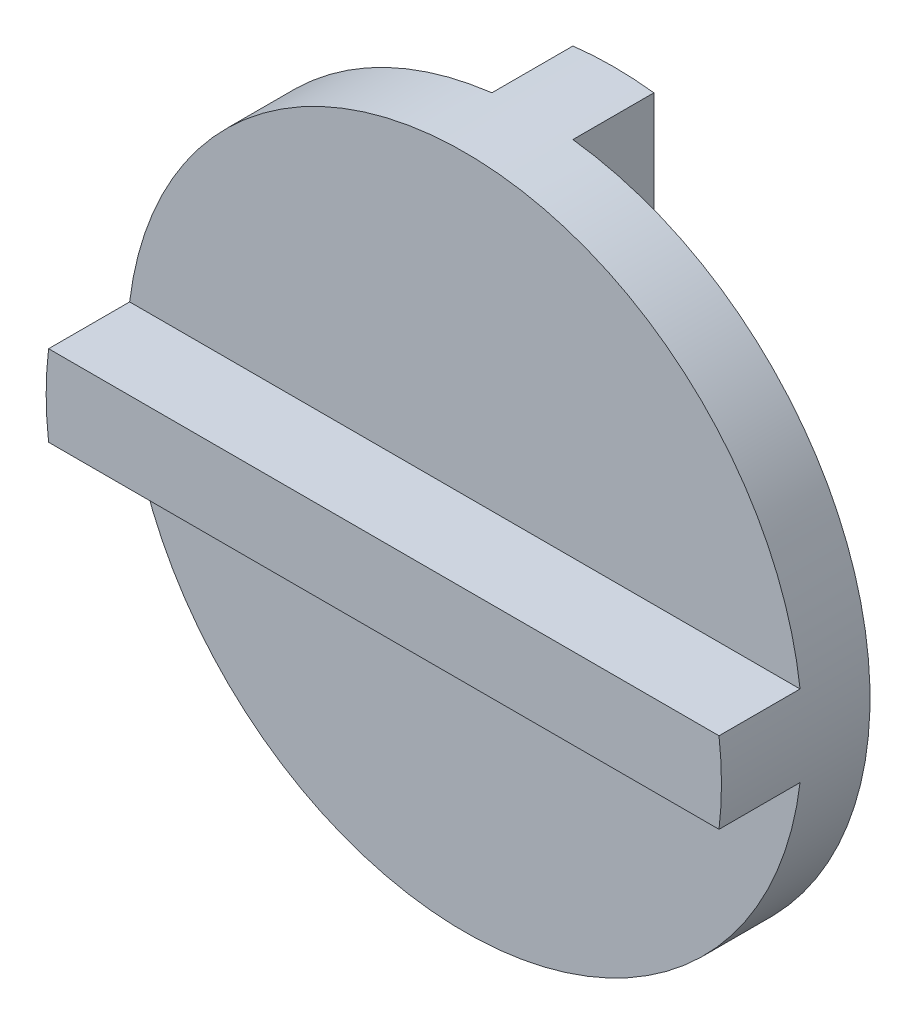
from build123d import *
from build123d.topology import SkipClean

# Parameters (mm, degrees)
DISC_PROFILE_100_R = 50
DISC_BODY_DEPTH    = 5
FACE_START         = 12
FACE_RIB_1_DEPTH   = 12
FACE_RIB_2_DEPTH   = 12


with BuildPart() as part:
    # Disc Profile Ø100 → Disc Body (new, symmetric)
    with BuildSketch(Plane.XY):
        Circle(DISC_PROFILE_100_R)
    extrude(amount=DISC_BODY_DEPTH, both=True)

    # Face Rib 1 Profile → Face Rib 1 (add)
    with SkipClean():  # the faces are left unmerged after this step: merging them gives an invalid solid
        with BuildSketch(Plane.XY.offset(5).offset(FACE_START)):
            with BuildLine():
                Line((49.638694584, -6), (-49.638694584, -6))
                ThreePointArc((-49.638694584, -6), (-50, 0), (-49.638694584, 6))
                Line((-49.638694584, 6), (49.638694584, 6))
                ThreePointArc((49.638694584, 6), (50, 0), (49.638694584, -6))
            make_face()
        extrude(amount=-FACE_RIB_1_DEPTH)

    # Face Rib 2 Profile → Face Rib 2 (add)
    with SkipClean():  # the faces are left unmerged after this step: merging them gives an invalid solid
        with BuildSketch(Plane(origin=(0, 0, -5), x_dir=(-1, 0, 0), z_dir=(0, 0, -1))):
            with BuildLine():
                Line((-6, -49.638694584), (-6, 49.638694584))
                ThreePointArc((-6, 49.638694584), (0, 50), (6, 49.638694584))
                Line((6, 49.638694584), (6, -49.638694584))
                ThreePointArc((6, -49.638694584), (0, -50), (-6, -49.638694584))
            make_face()
        extrude(amount=FACE_RIB_2_DEPTH)


solid = part.part
